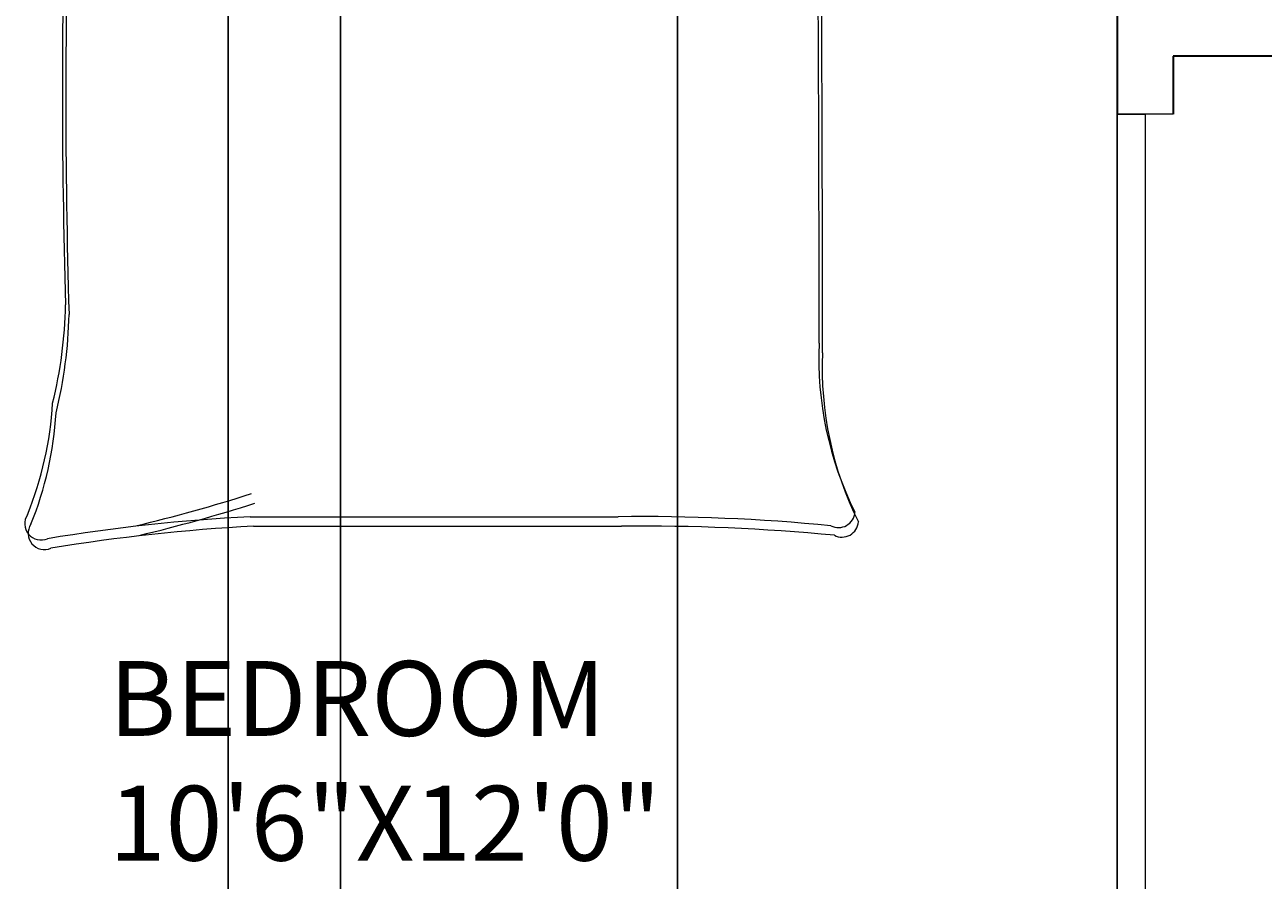
# Model space of a CAD drawing. Units: inches. Extents: x 1088 to 1703, y 668 to 1875.
# Tile 39 of 45: x 1498 to 1598, y 1675 to 1743. Entities that reach past the tile are written whole.
import ezdxf

# ---------------------------------------------------------------- set-up
doc = ezdxf.new("R2010")
doc.units = ezdxf.units.IN
for name, color, linetype, lineweight in [('A-ANNO-DIMS', 2, 'Continuous', 18), ('A-AREA-IDEN', 7, 'Continuous', 18), ('A-DOOR', 4, 'Continuous', 18), ('A-FURN', 8, 'Continuous', 13), ('A-WALL', 7, 'Continuous', 35)]:
    doc.layers.add(name, color=color, linetype=linetype, lineweight=lineweight)
doc.styles.get("Standard").update_dxf_attribs({"font": 'arial.ttf'})
doc.dimstyles.get("Standard").update_dxf_attribs({"dimtxt": 0.18, "dimasz": 0.18, "dimexe": 0.18, "dimexo": 0.0625, "dimgap": 0.09, "dimtad": 0, "dimtih": 1, "dimtoh": 1, "dimdec": 4, "dimzin": 0, "dimdsep": 46, "dimtxsty": 'Standard', "dimcen": 0.09, "dimadec": 0, "dimazin": 0, "dimtfac": 1, "dimtdec": 4, "dimtofl": 0, "dimtmove": 0, "dimatfit": 3, "dimfxl": 1, "dimtolj": 1, "dimtzin": 0, "dimarcsym": 0})

# ---------------------------------------------------------------- blocks, each defined once
blk = doc.blocks.new('BED-DOUBLE')
for p, q in [((95.77, 18.333), (95.77, 47.841)), ((95.003, 18.059), (95.003, 47.568))]:
    blk.add_line(p, q)
for centre, radius, start, end in [((82.321, 91.302), 27.652, 267.47136, 296.46809), ((83.088, 91.576), 27.652, 267.47136, 296.46809), ((94.554, 65.23), 1.322, 332.65876, 86.02002), ((95.32, 65.504), 1.322, 332.65876, 86.02002), ((254.489, 49.336), 159.496, 174.4998, 180.63509), ((255.256, 49.609), 159.496, 174.4998, 180.63509), ((81.308, -5405.342), 5469.019, 90.002168, 90.286887), ((82.075, -5405.068), 5469.019, 90.002168, 90.286887), ((-28.427, -20.646), 127.629, 13.38322, 17.70533), ((-27.661, -20.372), 127.629, 13.38322, 17.70533), ((240.775, 25.688), 145.971, 182.99578, 189.40907), ((241.542, 25.962), 145.971, 182.99578, 189.40907), ((60.679, 581.233), 578.221, 268.227709, 271.718541), ((61.445, 581.507), 578.221, 268.227709, 271.718541), ((77.344, -32.248), 35.527, 76.06484, 88.91125), ((78.111, -31.975), 35.527, 76.06484, 88.91125), ((84.25, -25.966), 28.247, 67.97508, 86.652), ((85.017, -25.693), 28.247, 67.97508, 86.652), ((96.337, 1.578), 1.306, 236.17358, 23.47814), ((95.57, 1.304), 1.306, 236.17358, 23.47814)]:
    blk.add_arc(centre, radius, start, end)
blk = doc.blocks.new('*D32')
at = {"layer": 'A-ANNO-DIMS', "color": 0, "lineweight": -2, "transparency": 16777216}
for p, q in [((1550.595, 1373.121), (1550.595, 1857.788)), ((1550.775, 1857.608), (1567.825, 1857.608)), ((1585.665, 1857.608), (1568.614, 1857.608)), ((1585.845, 1360.983), (1585.845, 1857.788))]:
    blk.add_line(p, q, dxfattribs=at)
at = {"layer": 'A-ANNO-DIMS', "color": 0, "transparency": 16777216}
for points in [[(1550.775, 1857.638), (1550.775, 1857.578), (1550.595, 1857.608)], [(1585.665, 1857.638), (1585.665, 1857.578), (1585.845, 1857.608)]]:
    blk.add_solid(points, dxfattribs=at)
at = {"layer": 'Defpoints', "color": 0, "transparency": 16777216}
for p in [(1585.845, 1857.608), (1550.595, 1373.058), (1585.845, 1360.921)]:
    blk.add_point(p, dxfattribs=at)
at = {"layer": 'A-ANNO-DIMS', "color": 0, "transparency": 16777216, "insert": (1568.22, 1857.608), "char_height": 0.18, "attachment_point": 5}
blk.add_mtext('\\A1;35.25', dxfattribs=at)
blk = doc.blocks.new('*D33')
at = {"layer": 'A-ANNO-DIMS', "color": 0, "lineweight": -2, "transparency": 16777216}
for p, q in [((1514.595, 1355.648), (1514.595, 1857.788)), ((1514.775, 1857.608), (1518.946, 1857.608)), ((1523.415, 1857.608), (1519.244, 1857.608)), ((1523.595, 1331.121), (1523.595, 1857.788))]:
    blk.add_line(p, q, dxfattribs=at)
at = {"layer": 'A-ANNO-DIMS', "color": 0, "transparency": 16777216}
for points in [[(1514.775, 1857.638), (1514.775, 1857.578), (1514.595, 1857.608)], [(1523.415, 1857.638), (1523.415, 1857.578), (1523.595, 1857.608)]]:
    blk.add_solid(points, dxfattribs=at)
at = {"layer": 'Defpoints', "color": 0, "transparency": 16777216}
for p in [(1523.595, 1857.608), (1514.595, 1355.585), (1523.595, 1331.058)]:
    blk.add_point(p, dxfattribs=at)
at = {"layer": 'A-ANNO-DIMS', "color": 0, "transparency": 16777216, "insert": (1519.095, 1857.608), "char_height": 0.18, "attachment_point": 5}
blk.add_mtext('\\A1;9', dxfattribs=at)

msp = doc.modelspace()

# ---------------------------------------------------------------- linework, layer by layer
at = {"layer": 'A-DOOR'}
for p, q in [((1590.345, 1736.337), (1585.845, 1736.337)), ((1585.845, 1736.337), (1588.095, 1736.337)), ((1588.095, 1736.337), (1588.095, 1673.058))]:
    msp.add_line(p, q, dxfattribs=at)
at = {"layer": 'A-WALL'}
for p, q in [((1585.845, 1745.49), (1585.845, 1736.337)), ((1590.345, 1740.99), (1590.345, 1736.337)), ((1620.345, 1740.99), (1590.345, 1740.99))]:
    msp.add_line(p, q, dxfattribs=at)

# ---------------------------------------------------------------- block references
at = {"layer": 'A-FURN', "rotation": 270}
msp.add_blockref('BED-DOUBLE', (1498.281, 1799.058), dxfattribs=at)

# ---------------------------------------------------------------- texts
at = {"layer": 'A-AREA-IDEN', "insert": (1505.032, 1692.478), "char_height": 6, "attachment_point": 1}
msp.add_mtext_dynamic_manual_height_columns('BEDROOM\\P10\'6"X12\'0"', width=157.49491, gutter_width=12.5, heights=[0], dxfattribs=at)

# ---------------------------------------------------------------- dimensions: what is measured, and where the dimension line sits
at = {"layer": 'A-ANNO-DIMS'}
for base, p1, p2, override, picture, middle in [((1523.595, 1857.608), (1514.595, 1355.585), (1523.595, 1331.058), {"dimdec": 0, "dimlfac": 1, "dimrnd": 0, "dimzin": 0, "dimdsep": 46, "dimlunit": 2}, '*D33', (1519.095, 1857.608)), ((1585.845, 1857.608), (1550.595, 1373.058), (1585.845, 1360.921), {"dimdec": 2, "dimlfac": 1, "dimrnd": 0, "dimzin": 0, "dimdsep": 46, "dimlunit": 2}, '*D32', (1568.22, 1857.608))]:
    dim = msp.add_linear_dim(base=base, p1=p1, p2=p2, dimstyle='Standard', override=override, dxfattribs=at)
    dim.commit()
    dim.dimension.update_dxf_attribs({"geometry": picture, "text_midpoint": middle})

doc.saveas('drawing.dxf')
